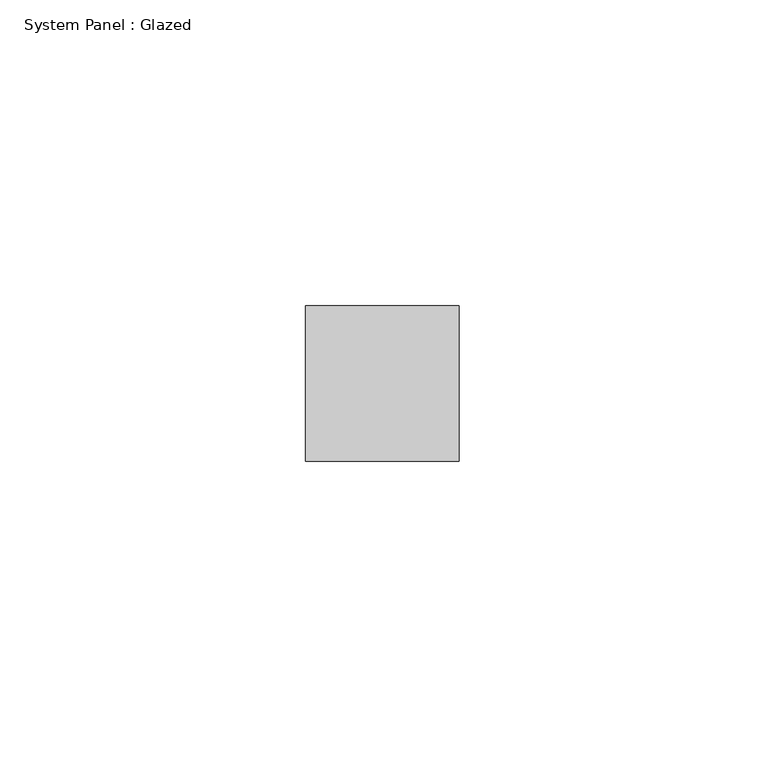
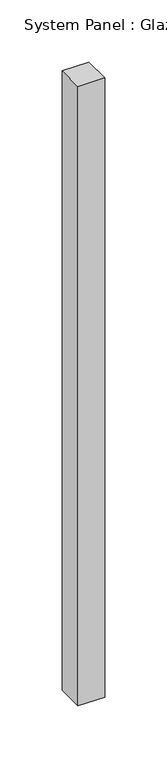
"""IFC4 building model written with IfcOpenShell, lengths in millimetres: plate geometry, System Panel : Glazed."""

from ifc_helpers import new_model, si_unit, origin, origin_with_axes, place, context, project, spatial, polyline, outline, extrude, source, transform, mapped, element, save


def system_panel_glazed_2900c437(model_context):
    return source(origin(), model_context, "Body", "SweptSolid", [
        extrude(outline(polyline([(12.5253346, 19.05), (-12.5253346, 19.05), (-12.5253346, 44.45), (12.5253346, 44.45), (12.5253346, 19.05)])), origin_with_axes(), (0.0, 0.0, 1.0), 609.6),
    ])


if __name__ == "__main__":
    model = new_model("IFC4")
    model_context = context("Model", 3, world=origin())
    ifc_project = project(units=[si_unit("LENGTHUNIT", "METRE", prefix="MILLI")], contexts=[model_context])
    site = spatial("IfcSite", under=ifc_project)
    building = spatial("IfcBuilding", under=site)
    placement = place(None, origin())
    system_panel_glazed_shape = system_panel_glazed_2900c437(model_context)
    element("IfcPlate", 1, ObjectType="System Panel : Glazed", at=placement, inside=building, context=model_context, shape_type="MappedRepresentation", body=[
        mapped(system_panel_glazed_shape, transform((0.0, 0.0, 0.0), x_axis=(1.0, 0.0, 0.0), y_axis=(0.0, 1.0, 0.0), z_axis=(0.0, 0.0, 1.0))),
    ])
    save(model, "model.ifc")

# Revit data of these elements
# Type "System Panel : Glazed"
#   Construction Type Id = "GSP4R"
#   Analytic Construction = "1/8 in Pilkington single glazing"
#   Visual Light Transmittance = 0.9
#   Solar Heat Gain Coefficient = 0.86
#   Heat Transfer Coefficient (U) = 1.18115 BTU/(h·ft²·°F)
# Element 1 (IfcPlate, "System Panel : Glazed")
#   Materials on its faces: "Glass"
# Materials
#   "Glass": class "Glass", colour RGB 0 128 192, transparency 0.75, Description = "Soda Lime Glass", Cost = 0
